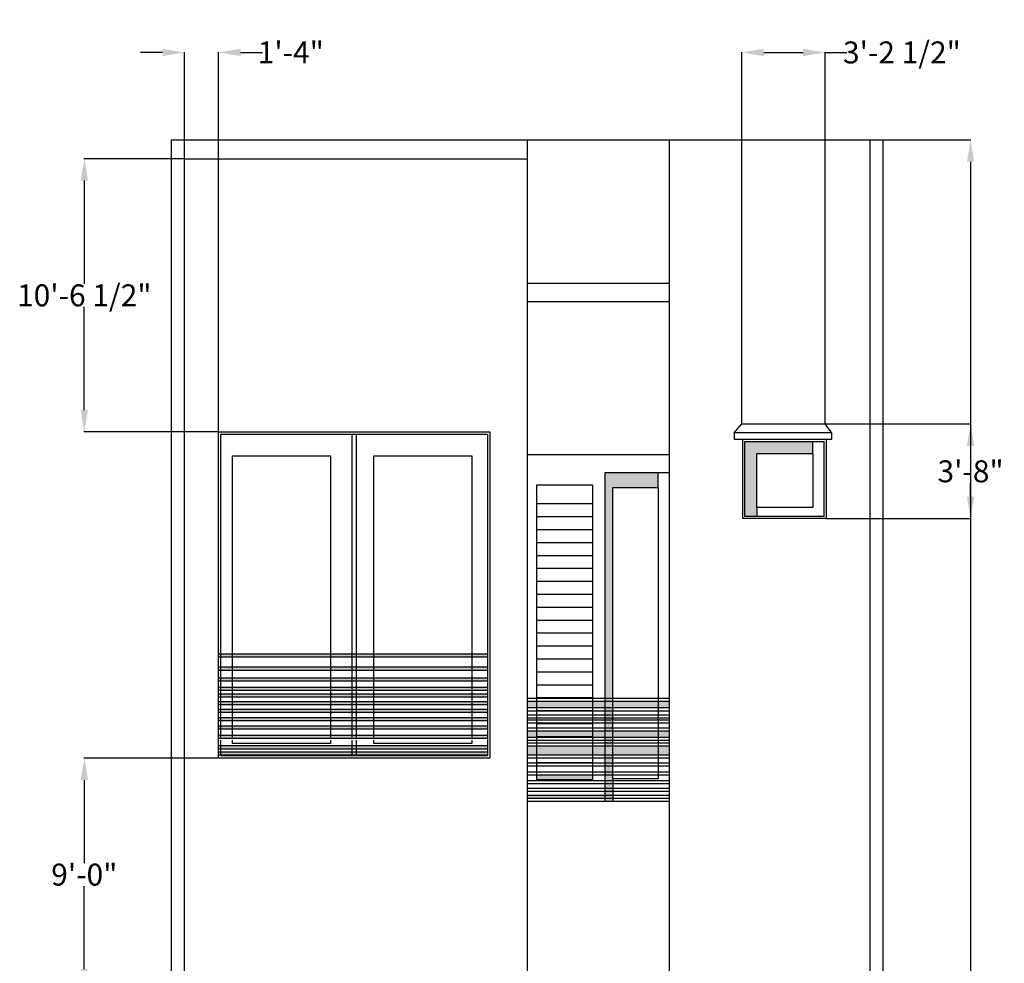
# Model space of a CAD drawing. Units: inches. Extents: x 41 to 5965, y 7 to 3328.
# Tile 5 of 6: x 4987 to 5444, y 2890 to 3328. Entities that reach past the tile are written whole.
import ezdxf

# ---------------------------------------------------------------- set-up
doc = ezdxf.new("R2010")
doc.units = ezdxf.units.IN
doc.header["$MEASUREMENT"] = 0
for name, color, linetype, lineweight in [('A-ANNO-DIMS', 2, 'Continuous', 18), ('A-ELEV', 7, 'Continuous', 25), ('A-ELEV-PATT', 8, 'Continuous', 13)]:
    doc.layers.add(name, color=color, linetype=linetype, lineweight=lineweight)
doc.styles.get("Standard").update_dxf_attribs({"font": 'arial.ttf'})
doc.dimstyles.get("Standard").update_dxf_attribs({"dimtxt": 10.18, "dimasz": 10.18, "dimexe": 0.18, "dimexo": 0.0625, "dimgap": 0.09, "dimtad": 0, "dimtih": 1, "dimtoh": 1, "dimdec": 0, "dimzin": 0, "dimdsep": 46, "dimlunit": 3, "dimtxsty": 'Standard', "dimcen": 0.09, "dimadec": 0, "dimazin": 0, "dimtfac": 1, "dimtdec": 0, "dimtofl": 0, "dimtmove": 0, "dimatfit": 3, "dimfxl": 1, "dimtolj": 1, "dimtzin": 0, "dimarcsym": 0})

# ---------------------------------------------------------------- blocks, each defined once
blk = doc.blocks.new('WIN-ELEV-1')
for p, q in [((0, 0), (0, 151.25)), ((0, 151.25), (125.74, 151.25)), ((125.74, 151.25), (125.74, 0)), ((1, 150.25), (124.74, 150.25)), ((1, 9.67), (1, 150.25)), ((124.74, 150.25), (124.74, 1)), ((1, 1), (1, 8.26)), ((125.74, 0), (0, 0)), ((124.74, 1), (1, 1))]:
    blk.add_line(p, q)
blk = doc.blocks.new('*D64')
at = {"layer": 'A-ANNO-DIMS', "color": 0, "lineweight": -2, "transparency": 16777216}
for p, q in [((5387.78, 3272.46), (5428.4, 3272.46)), ((5428.22, 3262.28), (5428.22, 2883.29)), ((5428.22, 2493.72), (5428.22, 2872.71)), ((5387.78, 2483.54), (5428.4, 2483.54))]:
    blk.add_line(p, q, dxfattribs=at)
at = {"layer": 'A-ANNO-DIMS', "color": 0, "transparency": 16777216}
for points in [[(5426.52, 3262.28), (5429.92, 3262.28), (5428.22, 3272.46)], [(5426.52, 2493.72), (5429.92, 2493.72), (5428.22, 2483.54)]]:
    blk.add_solid(points, dxfattribs=at)
at = {"layer": 'Defpoints', "color": 0, "transparency": 16777216}
for p in [(5387.72, 3272.46), (5428.22, 3272.46), (5387.72, 2483.54)]:
    blk.add_point(p, dxfattribs=at)
at = {"layer": 'A-ANNO-DIMS', "color": 0, "transparency": 16777216, "insert": (5428.22, 2878), "char_height": 10.18, "attachment_point": 5}
blk.add_mtext('\\A1;65\'-9"', dxfattribs=at)
blk = doc.blocks.new('*D72')
at = {"layer": 'A-ANNO-DIMS', "color": 0, "lineweight": -2, "transparency": 16777216}
for p, q in [((5079.42, 2985.67), (5017.04, 2985.67)), ((5017.22, 2975.49), (5017.22, 2936.92)), ((5017.22, 2887.76), (5017.22, 2926.34)), ((5082.94, 2877.58), (5017.04, 2877.58))]:
    blk.add_line(p, q, dxfattribs=at)
at = {"layer": 'A-ANNO-DIMS', "color": 0, "transparency": 16777216}
for points in [[(5015.52, 2975.49), (5018.92, 2975.49), (5017.22, 2985.67)], [(5015.52, 2887.76), (5018.92, 2887.76), (5017.22, 2877.58)]]:
    blk.add_solid(points, dxfattribs=at)
at = {"layer": 'Defpoints', "color": 0, "transparency": 16777216}
for p in [(5017.22, 2985.67), (5079.49, 2985.67), (5083, 2877.58)]:
    blk.add_point(p, dxfattribs=at)
at = {"layer": 'A-ANNO-DIMS', "color": 0, "transparency": 16777216, "insert": (5017.22, 2931.63), "char_height": 10.18, "attachment_point": 5}
blk.add_mtext('\\A1;9\'-0"', dxfattribs=at)
blk = doc.blocks.new('*D73')
at = {"layer": 'A-ANNO-DIMS', "color": 0, "lineweight": -2, "transparency": 16777216}
for p, q in [((5063.66, 3263.67), (5017.04, 3263.67)), ((5017.22, 3253.49), (5017.22, 3205.65)), ((5017.22, 3147.11), (5017.22, 3194.94)), ((5079.42, 3136.93), (5017.04, 3136.93))]:
    blk.add_line(p, q, dxfattribs=at)
at = {"layer": 'A-ANNO-DIMS', "color": 0, "transparency": 16777216}
for points in [[(5015.52, 3253.49), (5018.92, 3253.49), (5017.22, 3263.67)], [(5015.52, 3147.11), (5018.92, 3147.11), (5017.22, 3136.93)]]:
    blk.add_solid(points, dxfattribs=at)
at = {"layer": 'Defpoints', "color": 0, "transparency": 16777216}
for p in [(5017.22, 3263.67), (5063.72, 3263.67), (5079.49, 3136.93)]:
    blk.add_point(p, dxfattribs=at)
at = {"layer": 'A-ANNO-DIMS', "color": 0, "transparency": 16777216, "insert": (5017.22, 3200.3), "char_height": 10.18, "attachment_point": 5}
blk.add_mtext('\\A1;10\'-6 1/2"', dxfattribs=at)
blk = doc.blocks.new('*D74')
at = {"layer": 'A-ANNO-DIMS', "color": 0, "lineweight": -2, "transparency": 16777216}
for p, q in [((5053.54, 3312.96), (5043.36, 3312.96)), ((5063.72, 3263.73), (5063.72, 3313.14)), ((5079.49, 3136.99), (5079.49, 3313.14)), ((5089.67, 3312.96), (5099.85, 3312.96))]:
    blk.add_line(p, q, dxfattribs=at)
at = {"layer": 'A-ANNO-DIMS', "color": 0, "transparency": 16777216}
for points in [[(5053.54, 3314.66), (5053.54, 3311.27), (5063.72, 3312.96)], [(5089.67, 3314.66), (5089.67, 3311.27), (5079.49, 3312.96)]]:
    blk.add_solid(points, dxfattribs=at)
at = {"layer": 'Defpoints', "color": 0, "transparency": 16777216}
for p in [(5079.49, 3312.96), (5063.72, 3263.67), (5079.49, 3136.93)]:
    blk.add_point(p, dxfattribs=at)
at = {"layer": 'A-ANNO-DIMS', "color": 0, "transparency": 16777216, "insert": (5112.99, 3312.96), "char_height": 10.18, "attachment_point": 5}
blk.add_mtext('\\A1;1\'-4"', dxfattribs=at)
blk = doc.blocks.new('*D75')
at = {"layer": 'A-ANNO-DIMS', "color": 0, "lineweight": -2, "transparency": 16777216}
for p, q in [((5322.12, 3140.71), (5322.12, 3313.14)), ((5332.3, 3312.96), (5350.54, 3312.96)), ((5360.72, 3140.71), (5360.72, 3313.14)), ((5360.72, 3312.96), (5370.9, 3312.96))]:
    blk.add_line(p, q, dxfattribs=at)
at = {"layer": 'A-ANNO-DIMS', "color": 0, "transparency": 16777216}
for points in [[(5332.3, 3314.66), (5332.3, 3311.27), (5322.12, 3312.96)], [(5350.54, 3314.66), (5350.54, 3311.27), (5360.72, 3312.96)]]:
    blk.add_solid(points, dxfattribs=at)
at = {"layer": 'Defpoints', "color": 0, "transparency": 16777216}
for p in [(5360.72, 3312.96), (5322.12, 3140.64), (5360.72, 3140.64)]:
    blk.add_point(p, dxfattribs=at)
at = {"layer": 'A-ANNO-DIMS', "color": 0, "transparency": 16777216, "insert": (5396.38, 3312.96), "char_height": 10.18, "attachment_point": 5}
blk.add_mtext('\\A1;3\'-2 1/2"', dxfattribs=at)
blk = doc.blocks.new('*D76')
at = {"layer": 'A-ANNO-DIMS', "color": 0, "lineweight": -2, "transparency": 16777216}
for p, q in [((5360.78, 3140.64), (5428.4, 3140.64)), ((5428.22, 3130.46), (5428.22, 3123.97)), ((5428.22, 3106.9), (5428.22, 3113.39)), ((5361.27, 3096.72), (5428.4, 3096.72))]:
    blk.add_line(p, q, dxfattribs=at)
at = {"layer": 'A-ANNO-DIMS', "color": 0, "transparency": 16777216}
for points in [[(5426.52, 3130.46), (5429.92, 3130.46), (5428.22, 3140.64)], [(5426.52, 3106.9), (5429.92, 3106.9), (5428.22, 3096.72)]]:
    blk.add_solid(points, dxfattribs=at)
at = {"layer": 'Defpoints', "color": 0, "transparency": 16777216}
for p in [(5360.72, 3140.64), (5428.22, 3140.64), (5361.2, 3096.72)]:
    blk.add_point(p, dxfattribs=at)
at = {"layer": 'A-ANNO-DIMS', "color": 0, "transparency": 16777216, "insert": (5428.22, 3118.68), "char_height": 10.18, "attachment_point": 5}
blk.add_mtext('\\A1;3\'-8"', dxfattribs=at)

msp = doc.modelspace()

# ---------------------------------------------------------------- hatches: boundary and pattern name
at = {"layer": 'A-ELEV-PATT'}
h = msp.add_hatch(color=256, dxfattribs=at)
h.dxf.hatch_style = 1
h.paths.add_polyline_path([(5323.61, 3097.72), (5329.11, 3097.72), (5329.11, 3101.92), (5329.11, 3126.91), (5355.14, 3126.91), (5355.14, 3132.53), (5323.61, 3132.53)])
h = msp.add_hatch(color=256, dxfattribs=at)
h.dxf.hatch_style = 1
h.paths.add_polyline_path([(5283.31, 3117.91), (5258.54, 3117.91), (5258.54, 2965.62), (5262.29, 2965.62), (5262.29, 2976.12), (5262.29, 3111.19), (5283.31, 3111.19)])
h = msp.add_hatch(color=256, dxfattribs=at)
h.dxf.hatch_style = 1
h.paths.add_polyline_path([(5204.23, 3034), (5079.49, 3034), (5079.49, 3032.59), (5204.23, 3032.59)])
h = msp.add_hatch(color=256, dxfattribs=at)
h.dxf.hatch_style = 1
h.paths.add_polyline_path([(5204.23, 3027.93), (5079.49, 3027.93), (5079.49, 3026.52), (5204.23, 3026.52)])
h = msp.add_hatch(color=256, dxfattribs=at)
h.dxf.hatch_style = 1
h.paths.add_polyline_path([(5204.23, 3022.93), (5079.49, 3022.93), (5079.49, 3021.52), (5204.23, 3021.52)])
h = msp.add_hatch(color=256, dxfattribs=at)
h.dxf.hatch_style = 1
h.paths.add_polyline_path([(5204.23, 3018.64), (5079.49, 3018.64), (5079.49, 3017.23), (5204.23, 3017.23)])
h = msp.add_hatch(color=256, dxfattribs=at)
h.dxf.hatch_style = 1
h.paths.add_polyline_path([(5204.23, 3015.41), (5079.49, 3015.41), (5079.49, 3014.01), (5204.23, 3014.01)])
h = msp.add_hatch(color=256, dxfattribs=at)
h.dxf.hatch_style = 1
h.paths.add_polyline_path([(5204.23, 3011.99), (5079.49, 3011.99), (5079.49, 3010.58), (5204.23, 3010.58)])
h = msp.add_hatch(color=256, dxfattribs=at)
h.dxf.hatch_style = 1
h.paths.add_polyline_path([(5252.94, 2998.3), (5227.05, 2998.3), (5227.05, 2995.7), (5252.94, 2995.7)])
h.paths.add_polyline_path([(5227.05, 2998.3), (5222.72, 2998.3), (5222.72, 2995.4), (5227.05, 2995.4)])
h.paths.add_polyline_path([(5283.31, 2998.3), (5262.29, 2998.3), (5262.29, 2995.4), (5283.31, 2995.4)])
h.paths.add_polyline_path([(5258.54, 2998.3), (5252.94, 2998.3), (5252.94, 2995.4), (5258.54, 2995.4)])
h.paths.add_polyline_path([(5288.65, 2998.3), (5283.31, 2998.3), (5283.31, 2995.4), (5288.65, 2995.4)])
h.paths.add_polyline_path([(5283.31, 3012.12), (5262.29, 3012.12), (5262.29, 3009.07), (5283.31, 3009.07)])
h.paths.add_polyline_path([(5252.94, 3012.12), (5227.05, 3012.12), (5227.05, 3009.07), (5252.94, 3009.07)])
h.paths.add_polyline_path([(5258.54, 3012.12), (5252.94, 3012.12), (5252.94, 3009.07), (5258.54, 3009.07)])
h.paths.add_polyline_path([(5288.65, 3012.12), (5283.31, 3012.12), (5283.31, 3009.07), (5288.65, 3009.07)])
h.paths.add_polyline_path([(5227.05, 3012.12), (5222.72, 3012.12), (5222.72, 3009.07), (5227.05, 3009.07)])
h.paths.add_polyline_path([(5283.31, 2991.38), (5262.29, 2991.38), (5262.29, 2987.26), (5283.31, 2987.26)])
h = msp.add_hatch(color=256, dxfattribs=at)
h.dxf.hatch_style = 1
h.paths.add_polyline_path([(5204.23, 3008.33), (5079.49, 3008.33), (5079.49, 3006.93), (5204.23, 3006.93)])
h = msp.add_hatch(color=256, dxfattribs=at)
h.dxf.hatch_style = 1
h.paths.add_polyline_path([(5204.23, 3004.54), (5079.49, 3004.54), (5079.49, 3003.13), (5204.23, 3003.13)])
h = msp.add_hatch(color=256, dxfattribs=at)
h.dxf.hatch_style = 1
h.paths.add_polyline_path([(5204.23, 3000.62), (5079.49, 3000.62), (5079.49, 2999.21), (5204.23, 2999.21)])
h = msp.add_hatch(color=256, dxfattribs=at)
h.dxf.hatch_style = 1
h.paths.add_polyline_path([(5204.23, 2996.34), (5079.49, 2996.34), (5079.49, 2994.93), (5204.23, 2994.93)])
h = msp.add_hatch(color=256, dxfattribs=at)
h.dxf.hatch_style = 1
h.paths.add_polyline_path([(5204.23, 2991.44), (5079.49, 2991.44), (5079.49, 2990.04), (5204.23, 2990.04)])
h = msp.add_hatch(color=256, dxfattribs=at)
h.dxf.hatch_style = 1
h.paths.add_polyline_path([(5252.94, 2991.38), (5227.05, 2991.38), (5227.05, 2987.26), (5252.94, 2987.26)])
h.paths.add_polyline_path([(5227.05, 2991.38), (5222.72, 2991.38), (5222.72, 2987.26), (5227.05, 2987.26)])
h.paths.add_polyline_path([(5258.54, 2991.38), (5252.94, 2991.38), (5252.94, 2987.26), (5258.54, 2987.26)])
h.paths.add_polyline_path([(5288.65, 2991.38), (5283.31, 2991.38), (5283.31, 2987.26), (5288.65, 2987.26)])
h.paths.add_polyline_path([(5252.94, 2977.87), (5227.05, 2977.87), (5227.05, 2975.58), (5252.94, 2975.58)])
h.paths.add_polyline_path([(5258.54, 2968.53), (5222.72, 2968.53), (5222.72, 2967.12), (5258.54, 2967.12)])
h = msp.add_hatch(color=256, dxfattribs=at)
h.dxf.hatch_style = 1
h.paths.add_polyline_path([(5204.23, 2988.52), (5079.49, 2988.52), (5079.49, 2987.11), (5204.23, 2987.11)])

# ---------------------------------------------------------------- linework, layer by layer
at = {"layer": 'A-ELEV'}
for p, q in [((5057.72, 2483.54), (5057.72, 3272.46)), ((5057.72, 3272.46), (5387.72, 3272.46)), ((5222.72, 2682.95), (5222.72, 3272.46)), ((5288.65, 2708.16), (5288.65, 3272.46)), ((5288.65, 2965.62), (5288.65, 3272.46)), ((5381.72, 2483.54), (5381.72, 3272.46)), ((5387.72, 2483.54), (5387.72, 3272.46)), ((5063.72, 2483.54), (5063.72, 3263.67)), ((5063.72, 3263.67), (5222.72, 3263.67)), ((5222.72, 3205.92), (5288.65, 3205.92)), ((5222.72, 3197.46), (5288.65, 3197.46)), ((5318.61, 3136.59), (5322.12, 3140.64)), ((5322.12, 3140.64), (5360.72, 3140.64)), ((5363.89, 3136.59), (5360.72, 3140.64)), ((5141.36, 3135.93), (5141.36, 2995.34)), ((5143.36, 3135.93), (5143.36, 2995.34)), ((5355.14, 3126.91), (5355.14, 3132.53)), ((5222.72, 3126.42), (5288.65, 3126.42)), ((5288.65, 3117.91), (5258.54, 3117.91)), ((5258.54, 3117.91), (5258.54, 2965.62)), ((5283.31, 3111.19), (5283.31, 3117.91)), ((5227.05, 3103.7), (5252.94, 3103.7)), ((5329.11, 3101.92), (5329.11, 3097.72)), ((5227.05, 3097.7), (5252.94, 3097.7)), ((5227.05, 3091.7), (5252.94, 3091.7)), ((5227.05, 3085.7), (5252.94, 3085.7)), ((5227.05, 3079.7), (5252.94, 3079.7)), ((5227.05, 3073.7), (5252.94, 3073.7)), ((5227.05, 3067.7), (5252.94, 3067.7)), ((5227.05, 3061.7), (5252.94, 3061.7)), ((5227.05, 3055.7), (5252.94, 3055.7)), ((5227.05, 3049.7), (5252.94, 3049.7)), ((5227.05, 3043.7), (5252.94, 3043.7)), ((5227.05, 3037.7), (5252.94, 3037.7)), ((5079.49, 3034), (5204.23, 3034)), ((5079.49, 3032.59), (5204.23, 3032.59)), ((5079.49, 3027.93), (5204.23, 3027.93)), ((5227.05, 3031.7), (5252.94, 3031.7)), ((5079.49, 3026.52), (5204.23, 3026.52)), ((5079.49, 3022.93), (5204.23, 3022.93)), ((5227.05, 3025.7), (5252.94, 3025.7)), ((5079.49, 3021.52), (5204.23, 3021.52)), ((5079.49, 3018.64), (5204.23, 3018.64)), ((5227.05, 3019.7), (5252.94, 3019.7)), ((5079.49, 3017.23), (5204.23, 3017.23)), ((5079.49, 3015.41), (5204.23, 3015.41)), ((5079.49, 3014.01), (5204.23, 3014.01)), ((5227.05, 3013.7), (5252.94, 3013.7)), ((5079.49, 3011.99), (5204.23, 3011.99)), ((5079.49, 3010.58), (5204.23, 3010.58)), ((5222.72, 3013.53), (5288.65, 3013.53)), ((5222.72, 3012.12), (5288.65, 3012.12)), ((5222.72, 3009.07), (5288.65, 3009.07)), ((5079.49, 3008.33), (5204.23, 3008.33)), ((5079.49, 3006.93), (5204.23, 3006.93)), ((5079.49, 3004.54), (5204.23, 3004.54)), ((5222.72, 3007.66), (5288.65, 3007.66)), ((5222.72, 3005.69), (5288.65, 3005.69)), ((5227.05, 3007.7), (5252.94, 3007.7)), ((5079.49, 3003.13), (5204.23, 3003.13)), ((5079.49, 3000.62), (5204.23, 3000.62)), ((5222.72, 3004.29), (5288.65, 3004.29)), ((5222.72, 3003.39), (5288.65, 3003.39)), ((5222.72, 3001.98), (5288.65, 3001.98)), ((5227.05, 3001.7), (5252.94, 3001.7)), ((5079.49, 2999.21), (5204.23, 2999.21)), ((5079.49, 2996.34), (5204.23, 2996.34)), ((5222.72, 2999.7), (5288.65, 2999.7)), ((5222.72, 2998.3), (5288.65, 2998.3)), ((5222.72, 2995.4), (5288.65, 2995.4)), ((5227.05, 2995.7), (5252.94, 2995.7)), ((5079.49, 2994.93), (5204.23, 2994.93)), ((5079.49, 2991.44), (5204.23, 2991.44)), ((5141.36, 2993.93), (5141.36, 2986.67)), ((5143.36, 2993.93), (5143.36, 2986.67)), ((5222.72, 2994), (5288.65, 2994)), ((5222.72, 2992.79), (5288.65, 2992.79)), ((5222.72, 2991.38), (5288.65, 2991.38)), ((5079.49, 2990.04), (5204.23, 2990.04)), ((5079.49, 2988.52), (5204.23, 2988.52)), ((5079.49, 2987.11), (5204.23, 2987.11)), ((5222.72, 2987.26), (5288.65, 2987.26)), ((5222.72, 2985.86), (5288.65, 2985.86)), ((5222.72, 2983.42), (5288.65, 2983.42)), ((5222.72, 2982.02), (5288.65, 2982.02)), ((5227.05, 2983.7), (5252.94, 2983.7)), ((5222.72, 2979.28), (5288.65, 2979.28)), ((5222.72, 2977.87), (5288.65, 2977.87)), ((5222.72, 2975.28), (5288.65, 2975.28)), ((5222.72, 2973.88), (5288.65, 2973.88)), ((5262.29, 2976.12), (5262.29, 2965.62)), ((5222.72, 2971.75), (5288.65, 2971.75)), ((5222.72, 2970.34), (5288.65, 2970.34)), ((5222.72, 2968.53), (5288.65, 2968.53)), ((5222.72, 2967.12), (5288.65, 2967.12)), ((5222.72, 2965.62), (5288.65, 2965.62))]:
    msp.add_line(p, q, dxfattribs=at)
for points in [[(5318.61, 3133.53), (5318.61, 3133.53), (5363.89, 3133.53), (5363.89, 3133.53), (5363.89, 3136.59), (5363.89, 3136.59), (5318.61, 3136.59), (5318.61, 3136.59)], [(5322.61, 3133.53), (5322.61, 3133.53), (5361.2, 3133.53), (5361.2, 3133.53), (5361.2, 3096.72), (5361.2, 3096.72), (5322.61, 3096.72), (5322.61, 3096.72)], [(5323.61, 3132.53), (5360.2, 3132.53), (5360.2, 3097.72), (5323.61, 3097.72)], [(5329.11, 3126.91), (5329.11, 3126.91), (5355.14, 3126.91), (5355.14, 3126.91), (5355.14, 3101.92), (5355.14, 3101.92), (5329.11, 3101.92), (5329.11, 3101.92)], [(5227.05, 3112.45), (5227.05, 3112.45), (5252.94, 3112.45), (5252.94, 3112.45), (5252.94, 2975.58), (5252.94, 2975.58), (5227.05, 2975.58), (5227.05, 2975.58)], [(5262.29, 3111.19), (5262.29, 3111.19), (5283.31, 3111.19), (5283.31, 3111.19), (5283.31, 2976.12), (5283.31, 2976.12), (5262.29, 2976.12), (5262.29, 2976.12)]]:
    msp.add_lwpolyline(points, close=True, dxfattribs=at)
for points in [[(5085.94, 2995.34), (5085.94, 3125.91), (5085.94, 3125.91), (5131.36, 3125.91), (5131.36, 3125.91), (5131.36, 2995.34)], [(5151.45, 2995.34), (5151.45, 3125.91), (5151.45, 3125.91), (5196.87, 3125.91), (5196.87, 3125.91), (5196.87, 2995.34)], [(5131.36, 2993.93), (5131.36, 2992.45), (5131.36, 2992.45), (5085.94, 2992.45), (5085.94, 2992.45), (5085.94, 2993.93)], [(5196.87, 2993.93), (5196.87, 2992.45), (5196.87, 2992.45), (5151.45, 2992.45), (5151.45, 2992.45), (5151.45, 2993.93)]]:
    msp.add_lwpolyline(points, dxfattribs=at)

# ---------------------------------------------------------------- block references
msp.add_blockref('WIN-ELEV-1', (5079.49, 2985.67), dxfattribs=at)

# ---------------------------------------------------------------- dimensions: what is measured, and where the dimension line sits
at = {"layer": 'A-ANNO-DIMS'}
for base, p1, p2, picture, middle in [((5360.72, 3312.96), (5322.12, 3140.64), (5360.72, 3140.64), '*D75', (5396.38, 3312.96)), ((5079.49, 3312.96), (5063.72, 3263.67), (5079.49, 3136.93), '*D74', (5112.99, 3312.96))]:
    dim = msp.add_linear_dim(base=base, p1=p1, p2=p2, dimstyle='Standard', override={"dimdec": 1, "dimlfac": 1, "dimrnd": 0, "dimzin": 1, "dimdsep": 46, "dimlunit": 4, "dimfrac": 2}, dxfattribs=at)
    dim.commit()
    dim.dimension.update_dxf_attribs({"geometry": picture, "text_midpoint": middle})
for base, p1, p2, picture, middle in [((5428.22, 3272.46), (5387.72, 2483.54), (5387.72, 3272.46), '*D64', (5428.22, 2878)), ((5017.22, 3263.67), (5079.49, 3136.93), (5063.72, 3263.67), '*D73', (5017.22, 3200.3)), ((5428.22, 3140.64), (5361.2, 3096.72), (5360.72, 3140.64), '*D76', (5428.22, 3118.68)), ((5017.22, 2985.67), (5083, 2877.58), (5079.49, 2985.67), '*D72', (5017.22, 2931.63))]:
    dim = msp.add_linear_dim(base=base, p1=p1, p2=p2, angle=90, dimstyle='Standard', override={"dimdec": 1, "dimlfac": 1, "dimrnd": 0, "dimzin": 1, "dimdsep": 46, "dimlunit": 4, "dimfrac": 2}, dxfattribs=at)
    dim.commit()
    dim.dimension.update_dxf_attribs({"geometry": picture, "text_midpoint": middle})

doc.saveas('drawing.dxf')
